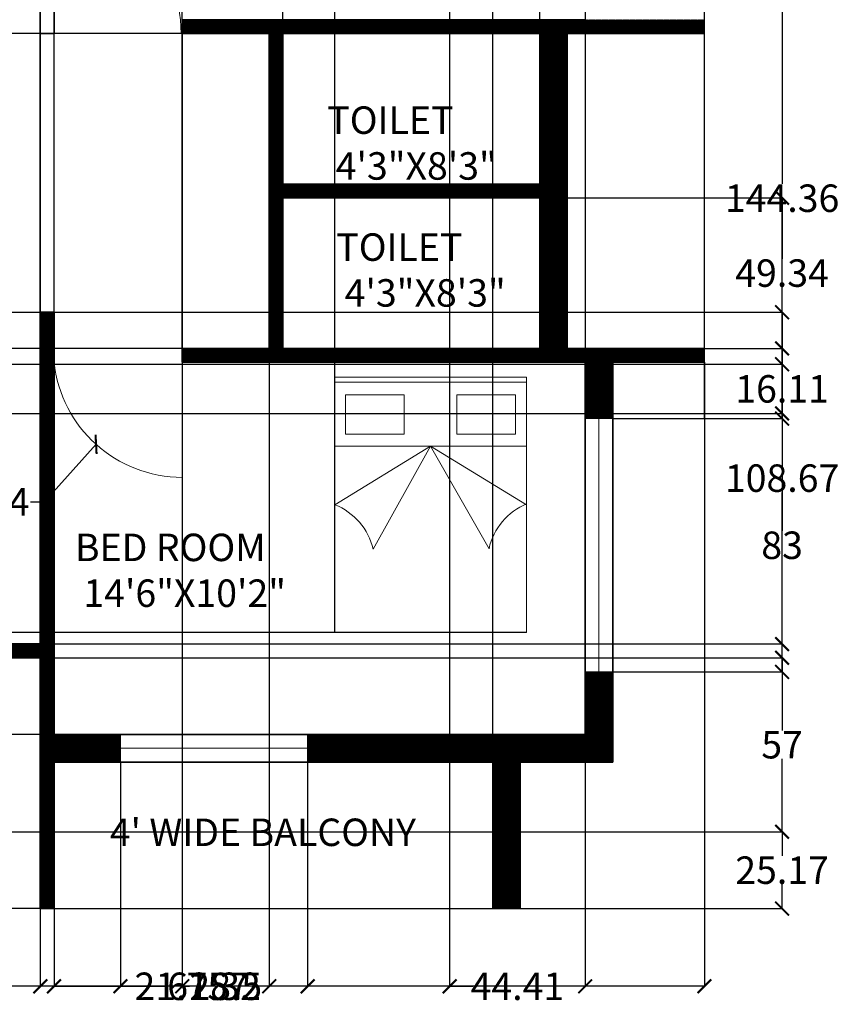
# Model space of a CAD drawing. Units: inches. Extents: x -43 to 552, y 22 to 537.
# Tile 3 of 4: x 283 to 552, y 28 to 351. Entities that reach past the tile are written whole.
import ezdxf

# ---------------------------------------------------------------- set-up
doc = ezdxf.new("R2010")
doc.units = ezdxf.units.IN
doc.header["$MEASUREMENT"] = 0
for name, color, linetype, lineweight in [('A-ANNO-DIMS', 2, 'Continuous', 18), ('A-AREA-IDEN', 7, 'Continuous', 18), ('A-DOOR', 4, 'Continuous', 18), ('A-FLOR', 7, 'Continuous', 25), ('A-FURN', 8, 'Continuous', 18), ('A-GLAZ', 4, 'Continuous', 18), ('A-WALL', 7, 'Continuous', 35), ('A-WALL-PATT', 252, 'Continuous', 13)]:
    doc.layers.add(name, color=color, linetype=linetype, lineweight=lineweight)
doc.styles.get("Standard").update_dxf_attribs({"font": 'arial.ttf'})
doc.dimstyles.get("Standard").update_dxf_attribs({"dimtxt": 9, "dimasz": 4.5, "dimexe": 0.18, "dimexo": 0.0625, "dimgap": 0.09, "dimtad": 0, "dimtih": 1, "dimtoh": 1, "dimdec": 1, "dimzin": 0, "dimdsep": 46, "dimlunit": 4, "dimtxsty": 'Standard', "dimblk": 'ARCHTICK', "dimcen": 0.09, "dimadec": 0, "dimazin": 0, "dimtfac": 1, "dimtdec": 1, "dimtofl": 0, "dimtmove": 0, "dimatfit": 3, "dimfxl": 1, "dimtolj": 1, "dimtzin": 0, "dimarcsym": 0})
pattern_1 = [(45, (-523.11303, 0), (-0.088388348, 0.088388348), [])]

# ---------------------------------------------------------------- blocks, each defined once
blk = doc.blocks.new('BED-DOUBLE')
for p, q in [((0, 83.65), (62.74, 83.65)), ((0, 0), (0, 83.65)), ((0, 81.91), (62.74, 81.91)), ((62.74, 83.65), (62.74, 0)), ((0, 61), (62.74, 61)), ((31.37, 61), (0, 41.83)), ((12.53, 27.23), (31.37, 61)), ((62.74, 41.83), (31.37, 61)), ((31.37, 61), (50.51, 27.4)), ((62.74, 0), (0, 0))]:
    blk.add_line(p, q)
for points in [[(3.55, 77.79), (22.76, 77.79), (22.76, 64.95), (3.55, 64.95)], [(59.19, 77.79), (39.98, 77.79), (39.98, 64.95), (59.19, 64.95)]]:
    blk.add_lwpolyline(points, close=True)
for centre, start, end in [((70.73, 22.94), 112.1918, 167.5578), ((-7.65, 22.59), 12.9482, 68.3142)]:
    blk.add_arc(centre, 20.7, start, end)
blk = doc.blocks.new('_ArchTick')
at = {"color": 0, "linetype": 'ByBlock', "const_width": 0.15}
blk.add_lwpolyline([(-0.5, -0.5), (0.5, 0.5)], dxfattribs=at)
blk = doc.blocks.new('*D8')
at = {"layer": 'A-ANNO-DIMS', "color": 0, "lineweight": -2, "transparency": 16777216}
for p, q in [((507.56, 238.71), (507.56, 34.14)), ((1.46, 84.88), (1.46, 34.14)), ((1.46, 34.32), (240.11, 34.32)), ((507.56, 34.32), (268.92, 34.32))]:
    blk.add_line(p, q, dxfattribs=at)
at = {"layer": 'Defpoints', "color": 0, "transparency": 16777216}
for p in [(507.56, 238.77), (1.46, 84.95), (507.56, 34.32)]:
    blk.add_point(p, dxfattribs=at)
at = {"layer": 'A-ANNO-DIMS', "color": 0, "lineweight": -2, "transparency": 16777216, "xscale": 4.5, "yscale": 4.5, "zscale": 4.5, "rotation": 180}
blk.add_blockref('_ArchTick', (1.46, 34.32), dxfattribs=at)
at = {"layer": 'A-ANNO-DIMS', "color": 0, "lineweight": -2, "transparency": 16777216, "xscale": 4.5, "yscale": 4.5, "zscale": 4.5}
blk.add_blockref('_ArchTick', (507.56, 34.32), dxfattribs=at)
at = {"layer": 'A-ANNO-DIMS', "color": 0, "transparency": 16777216, "insert": (254.51, 34.32), "char_height": 9, "attachment_point": 5}
blk.add_mtext('\\A1;506.1', dxfattribs=at)
blk = doc.blocks.new('*D9')
at = {"layer": 'A-ANNO-DIMS', "color": 0, "lineweight": -2, "transparency": 16777216}
for p, q in [((82.45, 505.95), (-24.17, 505.95)), ((-23.99, 505.95), (-23.99, 287.55)), ((-23.99, 59.77), (-23.99, 278.18)), ((289.95, 59.77), (-24.17, 59.77))]:
    blk.add_line(p, q, dxfattribs=at)
at = {"layer": 'Defpoints', "color": 0, "transparency": 16777216}
for p in [(-23.99, 505.95), (82.51, 505.95), (290.01, 59.77)]:
    blk.add_point(p, dxfattribs=at)
at = {"layer": 'A-ANNO-DIMS', "color": 0, "lineweight": -2, "transparency": 16777216, "xscale": 4.5, "yscale": 4.5, "zscale": 4.5}
for p, rotation in [((-23.99, 505.95), 90), ((-23.99, 59.77), 270)]:
    blk.add_blockref('_ArchTick', p, dxfattribs=dict(at, rotation=rotation))
at = {"layer": 'A-ANNO-DIMS', "color": 0, "transparency": 16777216, "insert": (-23.99, 282.86), "char_height": 9, "attachment_point": 5}
blk.add_mtext('\\A1;446.2', dxfattribs=at)
blk = doc.blocks.new('*D19')
at = {"layer": 'A-ANNO-DIMS', "color": 0, "lineweight": -2, "transparency": 16777216}
for p, q in [((507.62, 364.65), (533.19, 364.65)), ((533.01, 364.65), (533.01, 297.15)), ((533.01, 220.29), (533.01, 287.78)), ((507.62, 220.29), (533.19, 220.29))]:
    blk.add_line(p, q, dxfattribs=at)
at = {"layer": 'Defpoints', "color": 0, "transparency": 16777216}
for p in [(507.56, 364.65), (533.01, 364.65), (507.56, 220.29)]:
    blk.add_point(p, dxfattribs=at)
at = {"layer": 'A-ANNO-DIMS', "color": 0, "lineweight": -2, "transparency": 16777216, "xscale": 4.5, "yscale": 4.5, "zscale": 4.5}
for p, rotation in [((533.01, 364.65), 90), ((533.01, 220.29), 270)]:
    blk.add_blockref('_ArchTick', p, dxfattribs=dict(at, rotation=rotation))
at = {"layer": 'A-ANNO-DIMS', "color": 0, "transparency": 16777216, "insert": (533.01, 292.47), "char_height": 9, "attachment_point": 5}
blk.add_mtext('\\A1;144.36', dxfattribs=at)
blk = doc.blocks.new('*D20')
at = {"layer": 'A-ANNO-DIMS', "color": 0, "lineweight": -2, "transparency": 16777216}
for p, q in [((477.57, 220.29), (533.19, 220.29)), ((533.01, 220.29), (533.01, 183.47)), ((533.01, 137.29), (533.01, 174.1)), ((477.57, 137.29), (533.19, 137.29))]:
    blk.add_line(p, q, dxfattribs=at)
at = {"layer": 'Defpoints', "color": 0, "transparency": 16777216}
for p in [(477.51, 220.29), (533.01, 220.29), (477.51, 137.29)]:
    blk.add_point(p, dxfattribs=at)
at = {"layer": 'A-ANNO-DIMS', "color": 0, "lineweight": -2, "transparency": 16777216, "xscale": 4.5, "yscale": 4.5, "zscale": 4.5}
for p, rotation in [((533.01, 220.29), 90), ((533.01, 137.29), 270)]:
    blk.add_blockref('_ArchTick', p, dxfattribs=dict(at, rotation=rotation))
at = {"layer": 'A-ANNO-DIMS', "color": 0, "transparency": 16777216, "insert": (533.01, 178.79), "char_height": 9, "attachment_point": 5}
blk.add_mtext('\\A1;83', dxfattribs=at)
blk = doc.blocks.new('*D21')
at = {"layer": 'A-ANNO-DIMS', "color": 0, "lineweight": -2, "transparency": 16777216}
for p, q in [((290.07, 84.95), (533.19, 84.95)), ((533.01, 84.95), (533.01, 77.05)), ((533.01, 59.77), (533.01, 67.68)), ((290.07, 59.77), (533.19, 59.77))]:
    blk.add_line(p, q, dxfattribs=at)
at = {"layer": 'Defpoints', "color": 0, "transparency": 16777216}
for p in [(290.01, 84.95), (533.01, 84.95), (290.01, 59.77)]:
    blk.add_point(p, dxfattribs=at)
at = {"layer": 'A-ANNO-DIMS', "color": 0, "lineweight": -2, "transparency": 16777216, "xscale": 4.5, "yscale": 4.5, "zscale": 4.5}
for p, rotation in [((533.01, 84.95), 90), ((533.01, 59.77), 270)]:
    blk.add_blockref('_ArchTick', p, dxfattribs=dict(at, rotation=rotation))
at = {"layer": 'A-ANNO-DIMS', "color": 0, "transparency": 16777216, "insert": (533.01, 72.36), "char_height": 9, "attachment_point": 5}
blk.add_mtext('\\A1;25.17', dxfattribs=at)
blk = doc.blocks.new('*D24')
at = {"layer": 'A-ANNO-DIMS', "color": 0, "lineweight": -2, "transparency": 16777216}
for p, q in [((294.51, 107.71), (294.51, 34.14)), ((316.27, 107.71), (316.27, 34.14)), ((294.51, 34.32), (316.27, 34.32)), ((316.27, 34.32), (320.77, 34.32))]:
    blk.add_line(p, q, dxfattribs=at)
at = {"layer": 'Defpoints', "color": 0, "transparency": 16777216}
for p in [(294.51, 107.77), (316.27, 107.77), (316.27, 34.32)]:
    blk.add_point(p, dxfattribs=at)
at = {"layer": 'A-ANNO-DIMS', "color": 0, "lineweight": -2, "transparency": 16777216, "xscale": 4.5, "yscale": 4.5, "zscale": 4.5, "rotation": 180}
blk.add_blockref('_ArchTick', (294.51, 34.32), dxfattribs=at)
at = {"layer": 'A-ANNO-DIMS', "color": 0, "lineweight": -2, "transparency": 16777216, "xscale": 4.5, "yscale": 4.5, "zscale": 4.5}
blk.add_blockref('_ArchTick', (316.27, 34.32), dxfattribs=at)
at = {"layer": 'A-ANNO-DIMS', "color": 0, "transparency": 16777216, "insert": (339.62, 34.32), "char_height": 9, "attachment_point": 5}
blk.add_mtext('\\A1;21.757', dxfattribs=at)
blk = doc.blocks.new('*D25')
at = {"layer": 'A-ANNO-DIMS', "color": 0, "lineweight": -2, "transparency": 16777216}
for p, q in [((316.27, 107.71), (316.27, 34.14)), ((377.58, 107.71), (377.58, 34.14)), ((316.27, 34.32), (331.67, 34.32)), ((377.58, 34.32), (362.18, 34.32))]:
    blk.add_line(p, q, dxfattribs=at)
at = {"layer": 'Defpoints', "color": 0, "transparency": 16777216}
for p in [(316.27, 107.77), (377.58, 107.77), (377.58, 34.32)]:
    blk.add_point(p, dxfattribs=at)
at = {"layer": 'A-ANNO-DIMS', "color": 0, "lineweight": -2, "transparency": 16777216, "xscale": 4.5, "yscale": 4.5, "zscale": 4.5, "rotation": 180}
blk.add_blockref('_ArchTick', (316.27, 34.32), dxfattribs=at)
at = {"layer": 'A-ANNO-DIMS', "color": 0, "lineweight": -2, "transparency": 16777216, "xscale": 4.5, "yscale": 4.5, "zscale": 4.5}
blk.add_blockref('_ArchTick', (377.58, 34.32), dxfattribs=at)
at = {"layer": 'A-ANNO-DIMS', "color": 0, "transparency": 16777216, "insert": (346.93, 34.32), "char_height": 9, "attachment_point": 5}
blk.add_mtext('\\A1;61.32', dxfattribs=at)
blk = doc.blocks.new('*D28')
at = {"layer": 'A-ANNO-DIMS', "color": 0, "lineweight": -2, "transparency": 16777216}
for p, q in [((369.51, 297.17), (369.51, 531.58)), ((369.51, 531.4), (396.32, 531.4)), ((453.65, 531.4), (426.84, 531.4)), ((453.65, 297.17), (453.65, 531.58))]:
    blk.add_line(p, q, dxfattribs=at)
at = {"layer": 'Defpoints', "color": 0, "transparency": 16777216}
for p in [(453.65, 531.4), (369.51, 297.11), (453.65, 297.11)]:
    blk.add_point(p, dxfattribs=at)
at = {"layer": 'A-ANNO-DIMS', "color": 0, "lineweight": -2, "transparency": 16777216, "xscale": 4.5, "yscale": 4.5, "zscale": 4.5, "rotation": 180}
blk.add_blockref('_ArchTick', (369.51, 531.4), dxfattribs=at)
at = {"layer": 'A-ANNO-DIMS', "color": 0, "lineweight": -2, "transparency": 16777216, "xscale": 4.5, "yscale": 4.5, "zscale": 4.5}
blk.add_blockref('_ArchTick', (453.65, 531.4), dxfattribs=at)
at = {"layer": 'A-ANNO-DIMS', "color": 0, "transparency": 16777216, "insert": (411.58, 531.4), "char_height": 9, "attachment_point": 5}
blk.add_mtext('\\A1;84.14', dxfattribs=at)
blk = doc.blocks.new('*D29')
at = {"layer": 'A-ANNO-DIMS', "color": 0, "lineweight": -2, "transparency": 16777216}
for p, q in [((364.95, 346.45), (-24.17, 346.45)), ((-23.99, 346.45), (-23.99, 299.55)), ((-23.99, 243.27), (-23.99, 290.17)), ((364.95, 243.27), (-24.17, 243.27))]:
    blk.add_line(p, q, dxfattribs=at)
at = {"layer": 'Defpoints', "color": 0, "transparency": 16777216}
for p in [(-23.99, 346.45), (365.01, 346.45), (365.01, 243.27)]:
    blk.add_point(p, dxfattribs=at)
at = {"layer": 'A-ANNO-DIMS', "color": 0, "lineweight": -2, "transparency": 16777216, "xscale": 4.5, "yscale": 4.5, "zscale": 4.5}
for p, rotation in [((-23.99, 346.45), 90), ((-23.99, 243.27), 270)]:
    blk.add_blockref('_ArchTick', p, dxfattribs=dict(at, rotation=rotation))
at = {"layer": 'A-ANNO-DIMS', "color": 0, "transparency": 16777216, "insert": (-23.99, 294.86), "char_height": 9, "attachment_point": 5}
blk.add_mtext('\\A1;103.17', dxfattribs=at)
blk = doc.blocks.new('*D30')
at = {"layer": 'A-ANNO-DIMS', "color": 0, "lineweight": -2, "transparency": 16777216}
for p, q in [((369.57, 292.61), (533.19, 292.61)), ((533.01, 292.61), (533.01, 272.63)), ((533.01, 243.27), (533.01, 263.25)), ((369.57, 243.27), (533.19, 243.27))]:
    blk.add_line(p, q, dxfattribs=at)
at = {"layer": 'Defpoints', "color": 0, "transparency": 16777216}
for p in [(369.51, 292.61), (533.01, 292.61), (369.51, 243.27)]:
    blk.add_point(p, dxfattribs=at)
at = {"layer": 'A-ANNO-DIMS', "color": 0, "lineweight": -2, "transparency": 16777216, "xscale": 4.5, "yscale": 4.5, "zscale": 4.5}
for p, rotation in [((533.01, 292.61), 90), ((533.01, 243.27), 270)]:
    blk.add_blockref('_ArchTick', p, dxfattribs=dict(at, rotation=rotation))
at = {"layer": 'A-ANNO-DIMS', "color": 0, "transparency": 16777216, "insert": (533.01, 267.94), "char_height": 9, "attachment_point": 5}
blk.add_mtext('\\A1;49.34', dxfattribs=at)
blk = doc.blocks.new('*D32')
at = {"layer": 'A-ANNO-DIMS', "color": 0, "lineweight": -2, "transparency": 16777216}
for p, q in [((290.01, 255.18), (290.01, 531.58)), ((290.01, 531.4), (294.51, 531.4)), ((294.51, 255.18), (294.51, 531.58)), ((294.51, 531.4), (299.01, 531.4))]:
    blk.add_line(p, q, dxfattribs=at)
at = {"layer": 'Defpoints', "color": 0, "transparency": 16777216}
for p in [(294.51, 531.4), (290.01, 255.12), (294.51, 255.12)]:
    blk.add_point(p, dxfattribs=at)
at = {"layer": 'A-ANNO-DIMS', "color": 0, "lineweight": -2, "transparency": 16777216, "xscale": 4.5, "yscale": 4.5, "zscale": 4.5, "rotation": 180}
blk.add_blockref('_ArchTick', (290.01, 531.4), dxfattribs=at)
at = {"layer": 'A-ANNO-DIMS', "color": 0, "lineweight": -2, "transparency": 16777216, "xscale": 4.5, "yscale": 4.5, "zscale": 4.5}
blk.add_blockref('_ArchTick', (294.51, 531.4), dxfattribs=at)
at = {"layer": 'A-ANNO-DIMS', "color": 0, "transparency": 16777216, "insert": (307.51, 531.4), "char_height": 9, "attachment_point": 5}
blk.add_mtext('\\A1;4.5', dxfattribs=at)
blk = doc.blocks.new('*D33')
at = {"layer": 'A-ANNO-DIMS', "color": 0, "lineweight": -2, "transparency": 16777216}
for p, q in [((294.51, 59.84), (294.51, 531.58)), ((294.51, 531.4), (348.05, 531.4)), ((438.25, 531.4), (384.71, 531.4)), ((438.25, 59.84), (438.25, 531.58))]:
    blk.add_line(p, q, dxfattribs=at)
at = {"layer": 'Defpoints', "color": 0, "transparency": 16777216}
for p in [(438.25, 531.4), (294.51, 59.77), (438.25, 59.77)]:
    blk.add_point(p, dxfattribs=at)
at = {"layer": 'A-ANNO-DIMS', "color": 0, "lineweight": -2, "transparency": 16777216, "xscale": 4.5, "yscale": 4.5, "zscale": 4.5, "rotation": 180}
blk.add_blockref('_ArchTick', (294.51, 531.4), dxfattribs=at)
at = {"layer": 'A-ANNO-DIMS', "color": 0, "lineweight": -2, "transparency": 16777216, "xscale": 4.5, "yscale": 4.5, "zscale": 4.5}
blk.add_blockref('_ArchTick', (438.25, 531.4), dxfattribs=at)
at = {"layer": 'A-ANNO-DIMS', "color": 0, "transparency": 16777216, "insert": (366.38, 531.4), "char_height": 9, "attachment_point": 5}
blk.add_mtext('\\A1;143.74', dxfattribs=at)
blk = doc.blocks.new('*D34')
at = {"layer": 'A-ANNO-DIMS', "color": 0, "lineweight": -2, "transparency": 16777216}
for p, q in [((336.51, 346.38), (336.51, 34.14)), ((365.01, 346.38), (365.01, 34.14)), ((336.51, 34.32), (338.87, 34.32)), ((365.01, 34.32), (362.65, 34.32))]:
    blk.add_line(p, q, dxfattribs=at)
at = {"layer": 'Defpoints', "color": 0, "transparency": 16777216}
for p in [(336.51, 346.45), (365.01, 346.45), (365.01, 34.32)]:
    blk.add_point(p, dxfattribs=at)
at = {"layer": 'A-ANNO-DIMS', "color": 0, "lineweight": -2, "transparency": 16777216, "xscale": 4.5, "yscale": 4.5, "zscale": 4.5, "rotation": 180}
blk.add_blockref('_ArchTick', (336.51, 34.32), dxfattribs=at)
at = {"layer": 'A-ANNO-DIMS', "color": 0, "lineweight": -2, "transparency": 16777216, "xscale": 4.5, "yscale": 4.5, "zscale": 4.5}
blk.add_blockref('_ArchTick', (365.01, 34.32), dxfattribs=at)
at = {"layer": 'A-ANNO-DIMS', "color": 0, "transparency": 16777216, "insert": (350.76, 34.32), "char_height": 9, "attachment_point": 5}
blk.add_mtext('\\A1;28.5', dxfattribs=at)
blk = doc.blocks.new('*D35')
at = {"layer": 'A-ANNO-DIMS', "color": 0, "lineweight": -2, "transparency": 16777216}
for p, q in [((10.53, 141.95), (533.19, 141.95)), ((533.01, 141.95), (533.01, 118.11)), ((533.01, 84.95), (533.01, 108.78)), ((10.53, 84.95), (533.19, 84.95))]:
    blk.add_line(p, q, dxfattribs=at)
at = {"layer": 'Defpoints', "color": 0, "transparency": 16777216}
for p in [(10.46, 141.95), (533.01, 141.95), (10.46, 84.95)]:
    blk.add_point(p, dxfattribs=at)
at = {"layer": 'A-ANNO-DIMS', "color": 0, "lineweight": -2, "transparency": 16777216, "xscale": 4.5, "yscale": 4.5, "zscale": 4.5}
for p, rotation in [((533.01, 141.95), 90), ((533.01, 84.95), 270)]:
    blk.add_blockref('_ArchTick', p, dxfattribs=dict(at, rotation=rotation))
at = {"layer": 'A-ANNO-DIMS', "color": 0, "transparency": 16777216, "insert": (533.01, 113.45), "char_height": 9, "attachment_point": 5}
blk.add_mtext('\\A1;57', dxfattribs=at)
blk = doc.blocks.new('*D37')
at = {"layer": 'A-ANNO-DIMS', "color": 0, "lineweight": -2, "transparency": 16777216}
for p, q in [((248.01, 346.38), (248.01, 34.14)), ((290.01, 346.38), (290.01, 34.14)), ((248.01, 34.32), (262.34, 34.32)), ((290.01, 34.32), (275.68, 34.32))]:
    blk.add_line(p, q, dxfattribs=at)
at = {"layer": 'Defpoints', "color": 0, "transparency": 16777216}
for p in [(248.01, 346.45), (290.01, 346.45), (290.01, 34.32)]:
    blk.add_point(p, dxfattribs=at)
at = {"layer": 'A-ANNO-DIMS', "color": 0, "lineweight": -2, "transparency": 16777216, "xscale": 4.5, "yscale": 4.5, "zscale": 4.5, "rotation": 180}
blk.add_blockref('_ArchTick', (248.01, 34.32), dxfattribs=at)
at = {"layer": 'A-ANNO-DIMS', "color": 0, "lineweight": -2, "transparency": 16777216, "xscale": 4.5, "yscale": 4.5, "zscale": 4.5}
blk.add_blockref('_ArchTick', (290.01, 34.32), dxfattribs=at)
at = {"layer": 'A-ANNO-DIMS', "color": 0, "transparency": 16777216, "insert": (269.01, 34.32), "char_height": 9, "attachment_point": 5}
blk.add_mtext('\\A1;42', dxfattribs=at)
blk = doc.blocks.new('*D38')
at = {"layer": 'A-ANNO-DIMS', "color": 0, "lineweight": -2, "transparency": 16777216}
for p, q in [((294.51, 243.34), (294.51, 531.58)), ((294.51, 531.4), (308.84, 531.4)), ((336.51, 531.4), (322.18, 531.4)), ((336.51, 243.34), (336.51, 531.58))]:
    blk.add_line(p, q, dxfattribs=at)
at = {"layer": 'Defpoints', "color": 0, "transparency": 16777216}
for p in [(336.51, 531.4), (294.51, 243.27), (336.51, 243.27)]:
    blk.add_point(p, dxfattribs=at)
at = {"layer": 'A-ANNO-DIMS', "color": 0, "lineweight": -2, "transparency": 16777216, "xscale": 4.5, "yscale": 4.5, "zscale": 4.5, "rotation": 180}
blk.add_blockref('_ArchTick', (294.51, 531.4), dxfattribs=at)
at = {"layer": 'A-ANNO-DIMS', "color": 0, "lineweight": -2, "transparency": 16777216, "xscale": 4.5, "yscale": 4.5, "zscale": 4.5}
blk.add_blockref('_ArchTick', (336.51, 531.4), dxfattribs=at)
at = {"layer": 'A-ANNO-DIMS', "color": 0, "transparency": 16777216, "insert": (315.51, 531.4), "char_height": 9, "attachment_point": 5}
blk.add_mtext('\\A1;42', dxfattribs=at)
blk = doc.blocks.new('*D41')
at = {"layer": 'A-ANNO-DIMS', "color": 0, "lineweight": -2, "transparency": 16777216}
for p, q in [((468.51, 496.88), (468.51, 34.14)), ((424.1, 486.68), (424.1, 34.14)), ((424.1, 34.32), (431.72, 34.32)), ((468.51, 34.32), (460.89, 34.32))]:
    blk.add_line(p, q, dxfattribs=at)
at = {"layer": 'Defpoints', "color": 0, "transparency": 16777216}
for p in [(468.51, 496.95), (424.1, 486.74), (468.51, 34.32)]:
    blk.add_point(p, dxfattribs=at)
at = {"layer": 'A-ANNO-DIMS', "color": 0, "lineweight": -2, "transparency": 16777216, "xscale": 4.5, "yscale": 4.5, "zscale": 4.5, "rotation": 180}
blk.add_blockref('_ArchTick', (424.1, 34.32), dxfattribs=at)
at = {"layer": 'A-ANNO-DIMS', "color": 0, "lineweight": -2, "transparency": 16777216, "xscale": 4.5, "yscale": 4.5, "zscale": 4.5}
blk.add_blockref('_ArchTick', (468.51, 34.32), dxfattribs=at)
at = {"layer": 'A-ANNO-DIMS', "color": 0, "transparency": 16777216, "insert": (446.31, 34.32), "char_height": 9, "attachment_point": 5}
blk.add_mtext('\\A1;44.41', dxfattribs=at)
blk = doc.blocks.new('*D42')
at = {"layer": 'A-ANNO-DIMS', "color": 0, "lineweight": -2, "transparency": 16777216}
for p, q in [((294.51, 116.84), (294.51, 531.58)), ((294.51, 531.4), (325.22, 531.4)), ((386.5, 531.4), (355.79, 531.4)), ((386.5, 150.32), (386.5, 531.58))]:
    blk.add_line(p, q, dxfattribs=at)
at = {"layer": 'Defpoints', "color": 0, "transparency": 16777216}
for p in [(386.5, 531.4), (386.5, 150.25), (294.51, 116.77)]:
    blk.add_point(p, dxfattribs=at)
at = {"layer": 'A-ANNO-DIMS', "color": 0, "lineweight": -2, "transparency": 16777216, "xscale": 4.5, "yscale": 4.5, "zscale": 4.5, "rotation": 180}
blk.add_blockref('_ArchTick', (294.51, 531.4), dxfattribs=at)
at = {"layer": 'A-ANNO-DIMS', "color": 0, "lineweight": -2, "transparency": 16777216, "xscale": 4.5, "yscale": 4.5, "zscale": 4.5}
blk.add_blockref('_ArchTick', (386.5, 531.4), dxfattribs=at)
at = {"layer": 'A-ANNO-DIMS', "color": 0, "transparency": 16777216, "insert": (340.5, 531.4), "char_height": 9, "attachment_point": 5}
blk.add_mtext('\\A1;91.98', dxfattribs=at)
blk = doc.blocks.new('*D43')
at = {"layer": 'A-ANNO-DIMS', "color": 0, "lineweight": -2, "transparency": 16777216}
for p, q in [((449.17, 150.25), (-24.17, 150.25)), ((-23.99, 150.25), (-23.99, 138.2)), ((-23.99, 116.77), (-23.99, 128.83)), ((468.45, 116.77), (-24.17, 116.77))]:
    blk.add_line(p, q, dxfattribs=at)
at = {"layer": 'Defpoints', "color": 0, "transparency": 16777216}
for p in [(-23.99, 150.25), (449.23, 150.25), (468.51, 116.77)]:
    blk.add_point(p, dxfattribs=at)
at = {"layer": 'A-ANNO-DIMS', "color": 0, "lineweight": -2, "transparency": 16777216, "xscale": 4.5, "yscale": 4.5, "zscale": 4.5}
for p, rotation in [((-23.99, 150.25), 90), ((-23.99, 116.77), 270)]:
    blk.add_blockref('_ArchTick', p, dxfattribs=dict(at, rotation=rotation))
at = {"layer": 'A-ANNO-DIMS', "color": 0, "transparency": 16777216, "insert": (-23.99, 133.51), "char_height": 9, "attachment_point": 5}
blk.add_mtext('\\A1;33.48', dxfattribs=at)
blk = doc.blocks.new('*D45')
at = {"layer": 'A-ANNO-DIMS', "color": 0, "lineweight": -2, "transparency": 16777216}
for p, q in [((194.03, 255.12), (533.19, 255.12)), ((533.01, 255.12), (533.01, 205.47)), ((533.01, 146.45), (533.01, 196.1)), ((194.03, 146.45), (533.19, 146.45))]:
    blk.add_line(p, q, dxfattribs=at)
at = {"layer": 'Defpoints', "color": 0, "transparency": 16777216}
for p in [(193.96, 255.12), (533.01, 255.12), (193.96, 146.45)]:
    blk.add_point(p, dxfattribs=at)
at = {"layer": 'A-ANNO-DIMS', "color": 0, "lineweight": -2, "transparency": 16777216, "xscale": 4.5, "yscale": 4.5, "zscale": 4.5}
for p, rotation in [((533.01, 255.12), 90), ((533.01, 146.45), 270)]:
    blk.add_blockref('_ArchTick', p, dxfattribs=dict(at, rotation=rotation))
at = {"layer": 'A-ANNO-DIMS', "color": 0, "transparency": 16777216, "insert": (533.01, 200.78), "char_height": 9, "attachment_point": 5}
blk.add_mtext('\\A1;108.67', dxfattribs=at)
blk = doc.blocks.new('*D54')
at = {"layer": 'A-ANNO-DIMS', "color": 0, "lineweight": -2, "transparency": 16777216}
for p, q in [((185.87, 238.07), (533.19, 238.07)), ((533.01, 238.07), (533.01, 234.7)), ((533.01, 221.96), (533.01, 225.33)), ((185.87, 221.96), (533.19, 221.96))]:
    blk.add_line(p, q, dxfattribs=at)
at = {"layer": 'Defpoints', "color": 0, "transparency": 16777216}
for p in [(185.81, 238.07), (533.01, 238.07), (185.81, 221.96)]:
    blk.add_point(p, dxfattribs=at)
at = {"layer": 'A-ANNO-DIMS', "color": 0, "lineweight": -2, "transparency": 16777216, "xscale": 4.5, "yscale": 4.5, "zscale": 4.5}
for p, rotation in [((533.01, 238.07), 90), ((533.01, 221.96), 270)]:
    blk.add_blockref('_ArchTick', p, dxfattribs=dict(at, rotation=rotation))
at = {"layer": 'A-ANNO-DIMS', "color": 0, "transparency": 16777216, "insert": (533.01, 230.01), "char_height": 9, "attachment_point": 5}
blk.add_mtext('\\A1;16.11', dxfattribs=at)
blk = doc.blocks.new('*D55')
at = {"layer": 'A-ANNO-DIMS', "color": 0, "lineweight": -2, "transparency": 16777216}
for p, q in [((296.76, 416.65), (292.26, 416.65)), ((292.26, 416.65), (292.26, 390.33)), ((292.17, 346.45), (292.35, 346.45)), ((292.26, 346.36), (292.26, 346.54))]:
    blk.add_line(p, q, dxfattribs=at)
at = {"layer": 'Defpoints', "color": 0, "transparency": 16777216}
for p in [(292.26, 390.33), (292.26, 346.45)]:
    blk.add_point(p, dxfattribs=at)
at = {"layer": 'A-ANNO-DIMS', "color": 0, "lineweight": -2, "transparency": 16777216, "xscale": 4.5, "yscale": 4.5, "zscale": 4.5, "rotation": 269.9994946781158}
blk.add_blockref('_ArchTick', (292.26, 390.33), dxfattribs=at)
at = {"layer": 'A-ANNO-DIMS', "color": 0, "transparency": 16777216, "insert": (316.35, 416.65), "char_height": 9, "attachment_point": 5}
blk.add_mtext('\\A1;R43.88', dxfattribs=at)
blk = doc.blocks.new('*D57')
at = {"layer": 'A-ANNO-DIMS', "color": 0, "lineweight": -2, "transparency": 16777216}
for p, q in [((336.42, 243.27), (336.6, 243.27)), ((336.51, 243.18), (336.51, 243.36)), ((291.34, 193), (308.28, 211.86)), ((286.84, 193), (291.34, 193))]:
    blk.add_line(p, q, dxfattribs=at)
at = {"layer": 'Defpoints', "color": 0, "transparency": 16777216}
for p in [(336.51, 243.27), (308.28, 211.86)]:
    blk.add_point(p, dxfattribs=at)
at = {"layer": 'A-ANNO-DIMS', "color": 0, "lineweight": -2, "transparency": 16777216, "xscale": 4.5, "yscale": 4.5, "zscale": 4.5, "rotation": 48.05760462108148}
blk.add_blockref('_ArchTick', (308.28, 211.86), dxfattribs=at)
at = {"layer": 'A-ANNO-DIMS', "color": 0, "transparency": 16777216, "insert": (267.27, 193), "char_height": 9, "attachment_point": 5}
blk.add_mtext('\\A1;R42.24', dxfattribs=at)

msp = doc.modelspace()

# ---------------------------------------------------------------- hatches: boundary and pattern name
at = {"layer": 'A-WALL-PATT'}
h = msp.add_hatch(dxfattribs=at)
h.set_pattern_fill('ANSI31', color=256)
h.set_pattern_definition(pattern_1)
h.paths.add_polyline_path([(202.9985, 146.4471), (169.965, 146.4471), (169.965, 255.1157), (165.465, 255.1157), (165.465, 146.4471), (147.9805, 146.4471), (147.9805, 141.9471), (165.465, 141.9471), (165.465, 84.9471), (169.965, 84.9471), (169.965, 141.9471), (202.9985, 141.9471)])
h.paths.add_polyline_path([(294.5106, 146.4471), (294.5106, 238.775), (294.5106, 243.275), (294.5106, 255.1157), (290.0106, 255.1157), (290.0106, 146.4471), (247.8411, 146.4471), (247.8411, 141.9471), (290.0106, 141.9471), (290.0106, 93.9471), (290.0106, 59.775), (294.5106, 59.775), (294.5106, 77.3814), (294.5106, 93.9471), (294.5106, 107.775), (316.2676, 107.775), (316.2676, 116.775), (294.5106, 116.775)])
h.paths.add_polyline_path([(10.465, 346.4471), (82.5106, 346.4471), (91.5106, 346.4471), (91.5106, 358.2163), (82.5106, 358.2163), (82.5106, 350.9471), (1.465, 350.9471), (1.465, 84.9471), (10.465, 84.9471), (10.465, 141.9471), (56.4237, 141.9471), (56.4237, 146.4471), (10.465, 146.4471)])
h.paths.add_polyline_path([(91.5106, 496.9471), (107.5106, 496.9471), (107.5106, 505.9471), (82.5106, 505.9471), (82.5106, 400.4471), (147.5106, 400.4471), (147.5106, 346.4471), (248.0106, 346.4471), (248.0106, 350.9471), (152.0106, 350.9471), (152.0106, 496.9471), (197.0106, 496.9471), (197.0106, 505.9471), (131.5106, 505.9471), (131.5106, 496.9471), (147.5106, 496.9471), (147.5106, 404.9471), (91.5106, 404.9471)])
h.paths.add_polyline_path([(477.5106, 505.9471), (245.0106, 505.9471), (245.0106, 496.9471), (290.0106, 496.9471), (290.0106, 390.2693, -0.02565505), (294.5106, 390.2693), (294.5106, 496.9471), (468.5106, 496.9471), (468.5106, 460.1763), (477.5106, 460.1763)])
h = msp.add_hatch(dxfattribs=at)
h.set_pattern_fill('ANSI31', color=256)
h.set_pattern_definition(pattern_1)
h.paths.add_polyline_path([(462.6472, 350.9471), (453.6472, 350.9471), (453.6472, 243.275), (462.6472, 243.275)])
h.paths.add_polyline_path([(507.5611, 350.9471), (468.5106, 350.9471), (462.6472, 350.9471), (462.6472, 346.4471), (468.5106, 346.4471), (507.5611, 346.4471)])
h.paths.add_polyline_path([(453.6472, 350.9471), (336.5106, 350.9471), (336.5106, 346.4471), (453.6472, 346.4471)])
h.paths.add_polyline_path([(477.5106, 137.2859), (468.5106, 137.2859), (468.5106, 116.775), (377.5838, 116.775), (377.5838, 107.775), (438.2457, 107.775), (438.2457, 59.775), (447.2457, 59.775), (447.2457, 107.775), (477.5106, 107.775)])
h.paths.add_polyline_path([(477.5106, 379.5395), (468.5106, 379.5395), (468.5106, 364.6452), (477.5106, 364.6452)])
h.paths.add_polyline_path([(477.5106, 238.775), (468.5106, 238.775), (468.5106, 220.2859), (477.5106, 220.2859)])
h.paths.add_polyline_path([(507.5611, 243.275), (468.5106, 243.275), (462.6472, 243.275), (462.6472, 238.775), (468.5106, 238.775), (477.5106, 238.775), (507.5611, 238.775)])
h.paths.add_polyline_path([(462.6472, 243.275), (453.6472, 243.275), (453.6472, 238.775), (462.6472, 238.775)])
h.paths.add_polyline_path([(453.6472, 243.275), (369.5106, 243.275), (369.5106, 292.6111), (453.6472, 292.6111), (453.6472, 297.1111), (369.5106, 297.1111), (369.5106, 346.4471), (365.0106, 346.4471), (365.0106, 243.275), (336.5106, 243.275), (336.5106, 238.775), (453.6472, 238.775)])

# ---------------------------------------------------------------- linework, layer by layer
at = {"layer": 'A-DOOR'}
for p, q in [((290.0106, 346.4471), (248.0106, 346.4471)), ((248.0106, 346.4471), (294.5106, 346.4471)), ((294.5106, 346.4471), (336.5106, 346.4471)), ((336.5106, 243.275), (294.5106, 243.275)), ((336.5106, 243.275), (336.5106, 201.0346))]:
    msp.add_line(p, q, dxfattribs=at)
for centre, radius, start, end in [((292.2606, 346.4471), 43.8799, 0, 180), ((336.5106, 243.275), 42.2404, 186.115504, 270)]:
    msp.add_arc(centre, radius, start, end, dxfattribs=at)
at = {"layer": 'A-FLOR'}
for p, q in [((507.5611, 220.2859), (507.5611, 364.6452)), ((477.5106, 220.2859), (507.5611, 220.2859)), ((147.5106, 84.9471), (290.0106, 84.9471)), ((290.0106, 59.775), (447.2457, 59.775))]:
    msp.add_line(p, q, dxfattribs=at)
at = {"layer": 'A-GLAZ'}
for p, q in [((468.5106, 220.2859), (477.5106, 220.2859)), ((473.0106, 220.2859), (473.0106, 137.2859)), ((468.5106, 137.2859), (477.5106, 137.2859)), ((316.2676, 116.775), (316.2676, 107.775)), ((377.5838, 116.775), (377.5838, 107.775)), ((316.2676, 112.275), (377.5838, 112.275))]:
    msp.add_line(p, q, dxfattribs=at)
at = {"layer": 'A-WALL'}
for p, q in [((290.0106, 496.9471), (290.0106, 350.9471)), ((294.5106, 496.9471), (294.5106, 350.9471)), ((290.0106, 350.9471), (290.0106, 346.4471)), ((294.5106, 350.9471), (294.5106, 346.4471)), ((336.5106, 350.9471), (336.5106, 346.4471)), ((336.5106, 350.9471), (468.5106, 350.9471)), ((453.6472, 350.9471), (453.6472, 238.775)), ((462.6472, 350.9471), (462.6472, 238.775)), ((290.0106, 346.4471), (294.5106, 346.4471)), ((336.5106, 346.4471), (453.6472, 346.4471)), ((365.0106, 346.4471), (365.0106, 243.275)), ((369.5106, 346.4471), (369.5106, 297.1111)), ((462.6472, 346.4471), (468.5106, 346.4471)), ((468.5106, 346.4471), (507.5611, 346.4471)), ((453.6472, 297.1111), (369.5106, 297.1111)), ((453.6472, 292.6111), (369.5106, 292.6111)), ((369.5106, 292.6111), (369.5106, 243.275)), ((290.0106, 146.4471), (290.0106, 255.1157)), ((294.5106, 255.1157), (290.0106, 255.1157)), ((294.5106, 243.275), (294.5106, 255.1157)), ((294.5106, 243.275), (294.5106, 238.775)), ((336.5106, 243.275), (365.0106, 243.275)), ((336.5106, 243.275), (336.5106, 238.775)), ((369.5106, 243.275), (468.5106, 243.275)), ((468.5106, 243.275), (507.5611, 243.275)), ((294.5106, 146.4471), (294.5106, 238.775)), ((336.5106, 238.775), (468.5106, 238.775)), ((468.5106, 238.775), (468.5106, 116.775)), ((468.5106, 238.775), (507.5611, 238.775)), ((477.5106, 238.775), (477.5106, 107.775)), ((169.965, 146.4471), (290.0106, 146.4471)), ((294.5106, 146.4471), (294.5106, 116.775)), ((169.965, 141.9471), (290.0106, 141.9471)), ((290.0106, 141.9471), (290.0106, 93.9471)), ((294.5106, 116.775), (468.5106, 116.775)), ((294.5106, 107.775), (438.2457, 107.775)), ((294.5106, 107.775), (294.5106, 93.9471)), ((438.2457, 107.775), (438.2457, 59.775)), ((447.2457, 107.775), (447.2457, 59.775)), ((447.2457, 107.775), (477.5106, 107.775)), ((290.0106, 93.9471), (290.0106, 59.775)), ((294.5106, 93.9471), (294.5106, 77.3814)), ((294.5106, 77.3814), (294.5106, 59.775))]:
    msp.add_line(p, q, dxfattribs=at)

# ---------------------------------------------------------------- block references
at = {"layer": 'A-FURN'}
msp.add_blockref('BED-DOUBLE', (386.4952, 150.2529), dxfattribs=at)

# ---------------------------------------------------------------- texts
at = {"layer": 'A-AREA-IDEN', "char_height": 9, "attachment_point": 1}
for s, insert in [('TOILET\\P 4\'3"X8\'3"', (384.0391, 322.5371)), ('TOILET\\P 4\'3"X8\'3"', (386.9733, 280.9505)), ('BED ROOM\\P 14\'6"X10\'2"', (301.3633, 182.5923)), ("4' WIDE BALCONY", (312.7697, 89.2603))]:
    msp.add_mtext_dynamic_manual_height_columns(s, width=549.697564, gutter_width=1, heights=[0], dxfattribs=dict(at, insert=insert))

# ---------------------------------------------------------------- dimensions: what is measured, and where the dimension line sits
at = {"layer": 'A-ANNO-DIMS'}
for base, p1, p2, override, picture, middle in [((294.5106, 531.3971), (290.0106, 255.1157), (294.5106, 255.1157), {"dimdec": 1, "dimlfac": 1, "dimrnd": 0, "dimzin": 0, "dimdsep": 46, "dimlunit": 2}, '*D32', (307.5082, 531.3971)), ((438.2457, 531.3971), (294.5106, 59.775), (438.2457, 59.775), {"dimdec": 2, "dimlfac": 1, "dimrnd": 0, "dimzin": 0, "dimdsep": 46, "dimlunit": 2}, '*D33', (366.3781, 531.3971)), ((336.5106, 531.3971), (294.5106, 243.275), (336.5106, 243.275), {"dimdec": 0, "dimlfac": 1, "dimrnd": 0, "dimzin": 0, "dimdsep": 46, "dimlunit": 2}, '*D38', (315.5106, 531.3971)), ((386.4952, 531.3971), (294.5106, 116.775), (386.4952, 150.2529), {"dimdec": 2, "dimlfac": 1, "dimrnd": 0, "dimzin": 0, "dimdsep": 46, "dimlunit": 2}, '*D42', (340.5029, 531.3971)), ((453.6472, 531.3971), (369.5106, 297.1111), (453.6472, 297.1111), {"dimdec": 2, "dimlfac": 1, "dimrnd": 0, "dimzin": 0, "dimdsep": 46, "dimlunit": 2}, '*D28', (411.5789, 531.3971)), ((468.5106, 34.325), (424.1025, 486.7427), (468.5106, 496.9471), {"dimdec": 2, "dimlfac": 1, "dimrnd": 0, "dimzin": 0, "dimdsep": 46, "dimlunit": 2}, '*D41', (446.3066, 34.325)), ((290.0106, 34.325), (248.0106, 346.4471), (290.0106, 346.4471), {"dimdec": 0, "dimlfac": 1, "dimrnd": 0, "dimzin": 0, "dimdsep": 46, "dimlunit": 2}, '*D37', (269.0106, 34.325)), ((365.0106, 34.325), (336.5106, 346.4471), (365.0106, 346.4471), {"dimdec": 1, "dimlfac": 1, "dimrnd": 0, "dimzin": 0, "dimdsep": 46, "dimlunit": 2}, '*D34', (350.7606, 34.325)), ((507.5611, 34.325), (1.465, 84.9471), (507.5611, 238.775), {"dimdec": 1, "dimlfac": 1, "dimrnd": 0, "dimzin": 0, "dimdsep": 46, "dimlunit": 2}, '*D8', (254.513, 34.325)), ((316.2676, 34.325), (294.5106, 107.775), (316.2676, 107.775), {"dimdec": 3, "dimlfac": 1, "dimrnd": 0, "dimzin": 0, "dimdsep": 46, "dimlunit": 2}, '*D24', (339.6158, 34.325)), ((377.5838, 34.325), (316.2676, 107.775), (377.5838, 107.775), {"dimdec": 2, "dimlfac": 1, "dimrnd": 0, "dimzin": 0, "dimdsep": 46, "dimlunit": 2}, '*D25', (346.9257, 34.325))]:
    dim = msp.add_linear_dim(base=base, p1=p1, p2=p2, dimstyle='Standard', override=override, dxfattribs=at)
    dim.commit()
    dim.dimension.update_dxf_attribs({"geometry": picture, "text_midpoint": middle})
for base, p1, p2, override, picture, middle in [((-23.985, 505.9471), (290.0106, 59.775), (82.5106, 505.9471), {"dimdec": 1, "dimlfac": 1, "dimrnd": 0, "dimzin": 0, "dimdsep": 46, "dimlunit": 2}, '*D9', (-23.985, 282.8611)), ((533.0111, 364.6452), (507.5611, 220.2859), (507.5611, 364.6452), {"dimdec": 2, "dimlfac": 1, "dimrnd": 0, "dimzin": 0, "dimdsep": 46, "dimlunit": 2}, '*D19', (533.0111, 292.4656)), ((-23.985, 346.4471), (365.0106, 243.275), (365.0106, 346.4471), {"dimdec": 2, "dimlfac": 1, "dimrnd": 0, "dimzin": 0, "dimdsep": 46, "dimlunit": 2}, '*D29', (-23.985, 294.8611)), ((533.0111, 292.6111), (369.5106, 243.275), (369.5106, 292.6111), {"dimdec": 2, "dimlfac": 1, "dimrnd": 0, "dimzin": 0, "dimdsep": 46, "dimlunit": 2}, '*D30', (533.0111, 267.943)), ((533.0111, 255.1157), (193.965, 146.4471), (193.965, 255.1157), {"dimdec": 2, "dimlfac": 1, "dimrnd": 0, "dimzin": 0, "dimdsep": 46, "dimlunit": 2}, '*D45', (533.0111, 200.7814)), ((533.0111, 238.0655), (185.8076, 221.9554), (185.8076, 238.0655), {"dimdec": 2, "dimlfac": 1, "dimrnd": 0, "dimzin": 0, "dimdsep": 46, "dimlunit": 2}, '*D54', (533.0111, 230.0105)), ((533.0111, 220.2859), (477.5106, 137.2859), (477.5106, 220.2859), {"dimdec": 0, "dimlfac": 1, "dimrnd": 0, "dimzin": 0, "dimdsep": 46, "dimlunit": 2}, '*D20', (533.0111, 178.7859)), ((-23.985, 150.2529), (468.5106, 116.775), (449.2346, 150.2529), {"dimdec": 2, "dimlfac": 1, "dimrnd": 0, "dimzin": 0, "dimdsep": 46, "dimlunit": 2}, '*D43', (-23.985, 133.5139)), ((533.0111, 141.9471), (10.465, 84.9471), (10.465, 141.9471), {"dimdec": 0, "dimlfac": 1, "dimrnd": 0, "dimzin": 0, "dimdsep": 46, "dimlunit": 2}, '*D35', (533.0111, 113.4471)), ((533.0111, 84.9471), (290.0106, 59.775), (290.0106, 84.9471), {"dimdec": 2, "dimlfac": 1, "dimrnd": 0, "dimzin": 0, "dimdsep": 46, "dimlunit": 2}, '*D21', (533.0111, 72.3611))]:
    dim = msp.add_linear_dim(base=base, p1=p1, p2=p2, angle=90, dimstyle='Standard', override=override, dxfattribs=at)
    dim.commit()
    dim.dimension.update_dxf_attribs({"geometry": picture, "text_midpoint": middle})
for center, mpoint, picture, middle in [((292.2606, 346.4471), (292.261, 390.327), '*D55', (316.3523, 416.655)), ((336.5106, 243.275), (308.2779, 211.8558), '*D57', (267.2748, 193.0044))]:
    dim = msp.add_radius_dim(center=center, mpoint=mpoint, dimstyle='Standard', override={"dimdec": 2, "dimlfac": 1, "dimrnd": 0, "dimzin": 0, "dimdsep": 46, "dimlunit": 2}, dxfattribs=at)
    dim.commit()
    dim.dimension.update_dxf_attribs({"geometry": picture, "text_midpoint": middle, "dimtype": 164})

doc.saveas('drawing.dxf')
